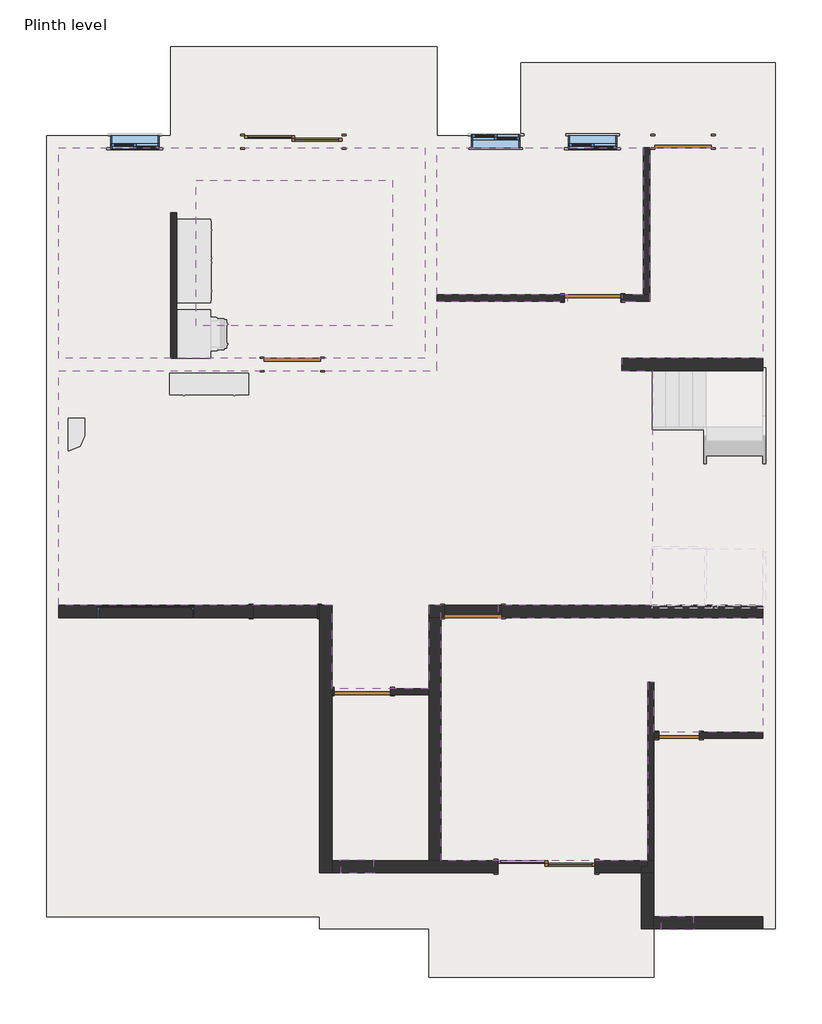
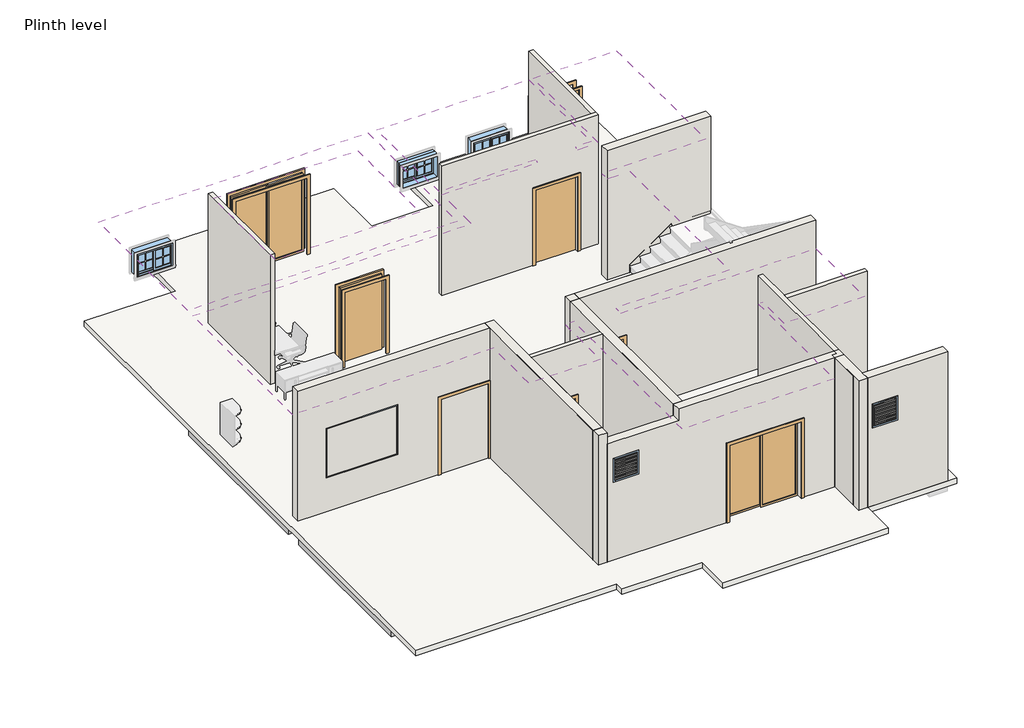
# One storey, part 1 of 2: 22 walls, 10 beams, 10 doors, 9 windows, 3 coverings, 1 slab.
"""IFC4 building model written with IfcOpenShell, lengths in millimetres."""

from ifc_helpers import new_model, si_unit, frame, origin, origin_with_axes, place, context, project, spatial, polyline, outline, extrude, faceted_brep, transform, mapped, element, save
from components import door_b7c0cbe2, door_d8f5dbb5, door_5f0ed9dd, door_edbf5142, door_f6232a3f, door_6982a541, window_dd9b4f56, window_f2d8fef0, window_5ed62b27

model = new_model("IFC4")

# Units and contexts
model_context = context("Model", 3, world=origin())
ifc_project = project(units=[si_unit("LENGTHUNIT", "METRE", prefix="MILLI")], contexts=[model_context])

# Site, building, storey
site = spatial("IfcSite", under=ifc_project)
building = spatial("IfcBuilding", under=site)
storey = spatial("IfcBuildingStorey", under=building, Name="Plinth level", Elevation=0.0)

# Beams
placement = place(None, origin())
element("IfcBeam", 1, ObjectType="Concrete-Rectangular Beam : 18X12", at=placement, inside=storey, context=model_context, shape_type="SweptSolid", body=[
    extrude(outline(polyline([(16230.9916032, -2769.6758122), (18402.6916032, -2769.6758122), (18402.6916032, -3226.8758122), (16688.1916032, -3226.8758122), (16688.1916032, -2998.2758122), (16230.9916032, -2998.2758122), (16230.9916032, -2769.6758122)])), frame((0.0, 0.0, -457.2), z_axis=(0.0, 0.0, 1.0), x_axis=(1.0, 0.0, 0.0)), (0.0, 0.0, 1.0), 304.8),
])
element("IfcBeam", 2, ObjectType="Concrete-Rectangular Beam : 18X12", at=placement, inside=storey, context=model_context, shape_type="Brep", body=[
    faceted_brep([(16230.9916032, -3226.8758122, -152.4), (16230.9916032, -2998.2758122, -152.4), (16230.9916032, -2769.6758122, -152.4), (12687.6916032, -2769.6758122, -152.4), (12687.6916032, -3226.8758122, -152.4), (16230.9916032, -3226.8758122, -457.2), (12687.6916032, -3226.8758122, -457.2), (16230.9916032, -2769.6758122, -457.2), (16230.9916032, -2998.2758122, -457.2), (12687.6916032, -2769.6758122, -457.2)], [[[0, 1, 2, 3, 4]], [[5, 0, 4, 6]], [[7, 8, 5, 6, 9]], [[2, 7, 9, 3]], [[3, 9, 6, 4]], [[2, 1, 0, 5, 8, 7]]]),
])
element("IfcBeam", 3, ObjectType="Concrete-Rectangular Beam : 18X12", at=placement, inside=storey, context=model_context, shape_type="Brep", body=[
    faceted_brep([(12459.0916032, -3226.8758122, -152.4), (12459.0916032, -2769.6758122, -152.4), (10858.8916032, -2769.6758122, -152.4), (10630.2916032, -2769.6758122, -152.4), (10630.2916032, -3226.8758122, -152.4), (12459.0916032, -2769.6758122, -457.2), (10858.8916032, -2769.6758122, -457.2), (10630.2916032, -2769.6758122, -457.2), (12459.0916032, -3226.8758122, -457.2), (10630.2916032, -3226.8758122, -457.2)], [[[0, 1, 2, 3, 4]], [[1, 5, 6, 7, 3, 2]], [[5, 8, 9, 7, 6]], [[8, 0, 4, 9]], [[0, 8, 5, 1]], [[4, 3, 7, 9]]]),
])
element("IfcBeam", 4, ObjectType="Concrete-Rectangular Beam : 18X12", at=placement, inside=storey, context=model_context, shape_type="Brep", body=[
    faceted_brep([(10858.8916032, -2769.6758122, -152.4), (10858.8916032, 1345.1241878, -152.4), (10858.8916032, 1802.3241878, -152.4), (10630.2916032, 1802.3241878, -152.4), (10630.2916032, 1345.1241878, -152.4), (10401.6916032, 1345.1241878, -152.4), (10401.6916032, -2769.6758122, -152.4), (10630.2916032, -2769.6758122, -152.4), (10858.8916032, 1802.3241878, -457.2), (10858.8916032, -2769.6758122, -457.2), (10858.8916032, 1345.1241878, -457.2), (10630.2916032, -2769.6758122, -457.2), (10401.6916032, -2769.6758122, -457.2), (10401.6916032, 1345.1241878, -457.2), (10630.2916032, 1345.1241878, -457.2), (10630.2916032, 1802.3241878, -457.2)], [[[0, 1, 2, 3, 4, 5, 6, 7]], [[8, 2, 1, 0, 9, 10]], [[8, 10, 9, 11, 12, 13, 14, 15]], [[12, 6, 5, 13]], [[0, 7, 6, 12, 11, 9]], [[2, 8, 15, 3]], [[14, 4, 3, 15]], [[4, 14, 13, 5]]]),
])
element("IfcBeam", 5, ObjectType="Concrete-Rectangular Beam : 18X12", at=placement, inside=storey, context=model_context, shape_type="Brep", body=[
    faceted_brep([(12459.0916032, 1345.1241878, -152.4), (12459.0916032, 1802.3241878, -152.4), (12153.8099466, 1802.3241878, -152.4), (10858.8916032, 1802.3241878, -152.4), (10858.8916032, 1345.1241878, -152.4), (12459.0916032, 1345.1241878, -457.2), (10858.8916032, 1345.1241878, -457.2), (12459.0916032, 1802.3241878, -457.2), (10858.8916032, 1802.3241878, -457.2), (12153.8099466, 1802.3241878, -457.2)], [[[0, 1, 2, 3, 4]], [[5, 0, 4, 6]], [[7, 5, 6, 8, 9]], [[1, 7, 9, 8, 3, 2]], [[4, 3, 8, 6]], [[1, 0, 5, 7]]]),
])
element("IfcBeam", 6, ObjectType="Concrete-Rectangular Beam : 18X12", at=placement, inside=storey, context=model_context, shape_type="Brep", body=[
    faceted_brep([(18402.6916032, 1345.1241878, -152.4), (18402.6916032, 1573.7241878, -152.4), (18402.6916032, 1802.3241878, -152.4), (12687.6916032, 1802.3241878, -152.4), (12687.6916032, 1345.1241878, -152.4), (18402.6916032, 1345.1241878, -457.2), (12687.6916032, 1345.1241878, -457.2), (18402.6916032, 1802.3241878, -457.2), (18402.6916032, 1573.7241878, -457.2), (12687.6916032, 1802.3241878, -457.2)], [[[0, 1, 2, 3, 4]], [[5, 0, 4, 6]], [[7, 8, 5, 6, 9]], [[2, 7, 9, 3]], [[3, 9, 6, 4]], [[2, 1, 0, 5, 8, 7]]]),
])
element("IfcBeam", 7, ObjectType="Concrete-Rectangular Beam : 18X12", at=placement, inside=storey, context=model_context, shape_type="Brep", body=[
    faceted_brep([(5601.0916032, 1802.3241878, -152.4), (5601.0916032, 1345.1241878, -152.4), (5829.6916032, 1345.1241878, -152.4), (10401.6916032, 1345.1241878, -152.4), (10401.6916032, 1802.3241878, -152.4), (5829.6916032, 1802.3241878, -152.4), (5601.0916032, 1345.1241878, -457.2), (5829.6916032, 1345.1241878, -457.2), (10401.6916032, 1345.1241878, -457.2), (5601.0916032, 1802.3241878, -457.2), (5829.6916032, 1802.3241878, -457.2), (10401.6916032, 1802.3241878, -457.2)], [[[0, 1, 2, 3, 4, 5]], [[1, 6, 7, 8, 3, 2]], [[6, 9, 10, 11, 8, 7]], [[9, 0, 5, 4, 11, 10]], [[1, 0, 9, 6]], [[4, 3, 8, 11]]]),
])
element("IfcBeam", 8, ObjectType="Concrete-Rectangular Beam : 18X12", at=placement, inside=storey, context=model_context, shape_type="Brep", body=[
    faceted_brep([(5601.0916032, -2769.6758122, -152.4), (5601.0916032, -3226.8758122, -152.4), (10401.6916032, -3226.8758122, -152.4), (10401.6916032, -2769.6758122, -152.4), (5829.6916032, -2769.6758122, -152.4), (5601.0916032, -3226.8758122, -457.2), (10401.6916032, -3226.8758122, -457.2), (5601.0916032, -2769.6758122, -457.2), (5829.6916032, -2769.6758122, -457.2), (10401.6916032, -2769.6758122, -457.2)], [[[0, 1, 2, 3, 4]], [[1, 5, 6, 2]], [[5, 7, 8, 9, 6]], [[7, 0, 4, 3, 9, 8]], [[1, 0, 7, 5]], [[3, 2, 6, 9]]]),
])
element("IfcBeam", 9, ObjectType="Concrete-Rectangular Beam : 18X12", at=placement, inside=storey, context=model_context, shape_type="Brep", body=[
    faceted_brep([(5829.6916032, 1345.1241878, -152.4), (5601.0916032, 1345.1241878, -152.4), (5372.4916032, 1345.1241878, -152.4), (5372.4916032, -2769.6758122, -152.4), (5601.0916032, -2769.6758122, -152.4), (5829.6916032, -2769.6758122, -152.4), (5829.6916032, 1345.1241878, -457.2), (5829.6916032, -2769.6758122, -457.2), (5372.4916032, 1345.1241878, -457.2), (5601.0916032, 1345.1241878, -457.2), (5601.0916032, -2769.6758122, -457.2), (5372.4916032, -2769.6758122, -457.2)], [[[0, 1, 2, 3, 4, 5]], [[6, 0, 5, 7]], [[8, 9, 6, 7, 10, 11]], [[2, 8, 11, 3]], [[2, 1, 0, 6, 9, 8]], [[5, 4, 3, 11, 10, 7]]]),
])
element("IfcBeam", 10, ObjectType="Concrete-Rectangular Beam : 18X12", at=placement, inside=storey, context=model_context, shape_type="Brep", body=[
    faceted_brep([(5829.6916032, 1802.3241878, -152.4), (5829.6916032, 6221.9241878, -152.4), (5829.6916032, 6679.1241878, -152.4), (5601.0916032, 6679.1241878, -152.4), (5601.0916032, 6221.9241878, -152.4), (5372.4916032, 6221.9241878, -152.4), (5372.4916032, 1802.3241878, -152.4), (5601.0916032, 1802.3241878, -152.4), (5372.4916032, 1802.3241878, -457.2), (5372.4916032, 6221.9241878, -457.2), (5829.6916032, 6679.1241878, -457.2), (5829.6916032, 6221.9241878, -457.2), (5829.6916032, 1802.3241878, -457.2), (5601.0916032, 1802.3241878, -457.2), (5601.0916032, 6221.9241878, -457.2), (5601.0916032, 6679.1241878, -457.2)], [[[0, 1, 2, 3, 4, 5, 6, 7]], [[8, 6, 5, 9]], [[10, 11, 12, 13, 8, 9, 14, 15]], [[10, 2, 1, 0, 12, 11]], [[0, 7, 6, 8, 13, 12]], [[2, 10, 15, 3]], [[14, 4, 3, 15]], [[4, 14, 9, 5]]]),
])

# Coverings
element("IfcCovering", 11, ObjectType="GWB on Mtl Stud", at=placement, inside=storey, context=model_context, shape_type="SweptSolid", body=[
    extrude(outline(polyline([(5486.7916032, 10412.9241878), (12382.4099466, 10412.9241878), (12382.4099466, 6450.5241878), (5486.7916032, 6450.5241878), (5486.7916032, 10412.9241878)]), holes=[polyline([(11772.8099466, 9803.3241878), (8077.5916032, 9803.3241878), (8077.5916032, 7060.1241878), (11772.8099466, 7060.1241878), (11772.8099466, 9803.3241878)])]), frame((0.0, 0.0, 2743.2), z_axis=(0.0, 0.0, 1.0), x_axis=(1.0, 0.0, 0.0)), (0.0, 0.0, 1.0), 107.95),
    extrude(outline(polyline([(11468.0099466, 9498.5241878), (11468.0099466, 7364.9241878), (8382.3916032, 7364.9241878), (8382.3916032, 9498.5241878), (11468.0099466, 9498.5241878)]), holes=[polyline([(11163.2099466, 9193.7241878), (8687.1916032, 9193.7241878), (8687.1916032, 8584.1241878), (11163.2099466, 8584.1241878), (11163.2099466, 9193.7241878)]), polyline([(8687.1916032, 8279.3241878), (8687.1916032, 7669.7241878), (11163.2099466, 7669.7241878), (11163.2099466, 8279.3241878), (8687.1916032, 8279.3241878)])]), frame((0.0, 0.0, 2743.2), z_axis=(0.0, 0.0, 1.0), x_axis=(1.0, 0.0, 0.0)), (0.0, 0.0, 1.0), 107.95),
])
element("IfcCovering", 12, ObjectType="GWB on Mtl Stud", at=placement, inside=storey, context=model_context, shape_type="SweptSolid", body=[
    extrude(outline(polyline([(11772.8099466, 9803.3241878), (11772.8099466, 7060.1241878), (8077.5916032, 7060.1241878), (8077.5916032, 9803.3241878), (11772.8099466, 9803.3241878)])), frame((0.0, 0.0, 2844.8), z_axis=(0.0, 0.0, 1.0), x_axis=(1.0, 0.0, 0.0)), (0.0, 0.0, 1.0), 107.95),
])
element("IfcCovering", 13, ObjectType="GWB on Mtl Stud", at=placement, inside=storey, context=model_context, shape_type="SweptSolid", body=[
    extrude(outline(polyline([(16497.2099466, 10412.9241878), (16497.2099466, 7644.3241878), (16086.4502792, 7644.3241878), (16086.4502792, 7530.0241878), (16611.5099466, 7530.0241878), (16611.5099466, 10412.9241878), (18745.5916032, 10412.9241878), (18745.5916032, 7530.0241878), (18745.5916032, 6450.5241878), (16086.4502792, 6450.5241878), (16086.4502792, 6221.9241878), (16662.7916032, 6221.9241878), (16662.7916032, 5155.1241878), (16662.7916032, 2869.1241878), (16662.7916032, 1802.3241878), (13751.6300735, 1802.3241878), (13751.6300735, 1573.7241878), (18745.5916032, 1573.7241878), (18745.5916032, -585.2758122), (16688.1916032, -585.2758122), (16688.1916032, 354.5241878), (16573.8916032, 354.5241878), (16573.8916032, -2998.2758122), (12687.6916032, -2998.2758122), (12687.6916032, 1802.3241878), (12459.0916032, 1802.3241878), (12459.0916032, 240.2241878), (10629.8628274, 240.2241878), (10629.8628274, 1802.3241878), (5486.7916032, 1802.3241878), (5486.7916032, 6221.9241878), (12611.0099466, 6221.9241878), (12611.0099466, 7530.0241878), (15070.4502792, 7530.0241878), (15070.4502792, 7644.3241878), (12611.0099466, 7644.3241878), (12611.0099466, 10412.9241878), (16497.2099466, 10412.9241878)])), frame((0.0, 0.0, 2743.2), z_axis=(0.0, 0.0, 1.0), x_axis=(1.0, 0.0, 0.0)), (0.0, 0.0, 1.0), 107.95),
])

# Doors
door_shape = door_b7c0cbe2(model_context)
element("IfcDoor", 14, ObjectType="Door-Double-Sliding : 72\" x 82\"", at=placement, inside=storey, context=model_context, shape_type="MappedRepresentation", body=[
    mapped(door_shape, transform((14668.8916032, -3239.5758122, 0.0), x_axis=(1.0, 0.0, 0.0), y_axis=(0.0, 1.0, 0.0), z_axis=(0.0, 0.0, 1.0))),
])
element("IfcDoor", 15, ObjectType="Door-Double-Sliding : 72\" x 82\"", at=placement, inside=storey, context=model_context, shape_type="MappedRepresentation", body=[
    mapped(door_shape, transform((9905.9099466, 10400.2241878, 0.0), x_axis=(1.0, 0.0, 0.0), y_axis=(0.0, 1.0, 0.0), z_axis=(0.0, 0.0, 1.0))),
])
element("IfcDoor", 16, ObjectType="Door-Double-Sliding : 72\" x 82\"", at=placement, inside=storey, context=model_context, shape_type="MappedRepresentation", body=[
    mapped(door_shape, transform((14668.8916032, -3239.5758122, 0.0), x_axis=(1.0, 0.0, 0.0), y_axis=(0.0, 1.0, 0.0), z_axis=(0.0, 0.0, 1.0))),
])
door_2_shape = door_d8f5dbb5(model_context)
element("IfcDoor", 17, ObjectType="Single-Flush : 30\" x 80\"", at=placement, inside=storey, context=model_context, shape_type="MappedRepresentation", body=[
    mapped(door_2_shape, transform((17164.4416032, -642.4258122, 0.0), x_axis=(-1.0, 0.0, 0.0), y_axis=(0.0, -1.0, 0.0), z_axis=(0.0, 0.0, 1.0))),
])
door_3_shape = door_5f0ed9dd(model_context)
element("IfcDoor", 18, ObjectType="Single-Flush : 42\" x 80\"", at=placement, inside=storey, context=model_context, shape_type="MappedRepresentation", body=[
    mapped(door_3_shape, transform((11201.7916032, 183.0741878, 0.0), x_axis=(-1.0, 0.0, 0.0), y_axis=(0.0, -1.0, 0.0), z_axis=(0.0, 0.0, 1.0))),
])
element("IfcDoor", 19, ObjectType="Single-Flush : 42\" x 80\"", at=placement, inside=storey, context=model_context, shape_type="MappedRepresentation", body=[
    mapped(door_3_shape, transform((15538.3599466, 7587.1741878, 0.0), x_axis=(1.0, 0.0, 0.0), y_axis=(0.0, 1.0, 0.0), z_axis=(0.0, 0.0, 1.0))),
])
door_4_shape = door_edbf5142(model_context)
element("IfcDoor", 20, ObjectType="Single-Flush : 42\" x 80\"", at=placement, inside=storey, context=model_context, shape_type="MappedRepresentation", body=[
    mapped(door_4_shape, transform((13284.5916032, 1688.0241878, 0.0), x_axis=(-1.0, 0.0, 0.0), y_axis=(0.0, -1.0, 0.0), z_axis=(0.0, 0.0, 1.0))),
])
element("IfcDoor", 21, ObjectType="Single-Flush : 42\" x 80\"", at=placement, inside=storey, context=model_context, shape_type="MappedRepresentation", body=[
    mapped(door_4_shape, transform((17240.1599466, 10527.2241878, 0.0), x_axis=(-1.0, 0.0, 0.0), y_axis=(0.0, -1.0, 0.0), z_axis=(0.0, 0.0, 1.0))),
])
door_5_shape = door_f6232a3f(model_context)
element("IfcDoor", 22, ObjectType="Single-Flush : 42\" x 80\"", at=placement, inside=storey, context=model_context, shape_type="MappedRepresentation", body=[
    mapped(door_5_shape, transform((9886.8599466, 6336.2241878, 0.0), x_axis=(-1.0, 0.0, 0.0), y_axis=(0.0, -1.0, 0.0), z_axis=(0.0, 0.0, 1.0))),
])
door_6_shape = door_6982a541(model_context)
element("IfcDoor", 23, ObjectType="Single-Flush : 48\" x 80\" 2", at=placement, inside=storey, context=model_context, shape_type="MappedRepresentation", body=[
    mapped(door_6_shape, transform((9753.9916032, 1688.0241878, 0.0), x_axis=(-1.0, 0.0, 0.0), y_axis=(0.0, -1.0, 0.0), z_axis=(0.0, 0.0, 1.0))),
])

# Slab
element("IfcSlab", 24, ObjectType="Concrete Slab - 6\"", at=placement, inside=storey, context=model_context, shape_type="SweptSolid", body=[
    extrude(outline(polyline([(5258.1916032, 10641.5241878), (7594.5099466, 10641.5241878), (7594.5099466, 12317.9241878), (12611.0099466, 12317.9241878), (12611.0099466, 10641.5241878), (14192.2689416, 10641.5241878), (14192.2689416, 12013.1241878), (18974.1916032, 12013.1241878), (18974.1916032, 10641.5241878), (18974.1916032, -4280.9758122), (16688.1916032, -4280.9758122), (16688.1916032, -5195.3758122), (12459.0916032, -5195.3758122), (12459.0916032, -4280.9758122), (10401.6916032, -4280.9758122), (10401.6916032, -4052.3758122), (5258.1916032, -4052.3758122), (5258.1916032, 10641.5241878)])), frame((0.0, 0.0, -152.4), z_axis=(0.0, 0.0, 1.0), x_axis=(1.0, 0.0, 0.0)), (0.0, 0.0, 1.0), 152.4),
])

# Walls
element("IfcWall", 25, ObjectType="4.5\"", at=placement, inside=storey, context=model_context, shape_type="Brep", body=[
    faceted_brep([(16688.1916032, -2998.2758122, 0.0), (16688.1916032, -699.5758122, 0.0), (16688.1916032, -585.2758122, 0.0), (16688.1916032, 354.5241878, 0.0), (16688.1916032, 354.5241878, 3505.2), (16688.1916032, -585.2758122, 3505.2), (16688.1916032, -699.5758122, 3505.2), (16688.1916032, -2998.2758122, 3505.2), (16573.8916032, -2998.2758122, 0.0), (16573.8916032, -2998.2758122, 3505.2), (16573.8916032, 354.5241878, 3505.2), (16573.8916032, 354.5241878, 0.0)], [[[0, 1, 2, 3, 4, 5, 6, 7]], [[8, 9, 10, 11]], [[3, 2, 1, 0, 8, 11]], [[4, 3, 11, 10]], [[7, 6, 5, 4, 10, 9]], [[0, 7, 9, 8]]]),
])
element("IfcWall", 26, ObjectType="4.5\"", at=placement, inside=storey, context=model_context, shape_type="SweptSolid", body=[
    extrude(outline(polyline([(0.0, 10630.2916032), (0.0, 10668.3916032), (2032.0, 10668.3916032), (2032.0, 11735.1916032), (0.0, 11735.1916032), (0.0, 12459.0916032), (3505.2, 12459.0916032), (3505.2, 10630.2916032), (0.0, 10630.2916032)])), frame((0.0, 125.9241878, 0.0), z_axis=(0.0, 1.0, 0.0), x_axis=(0.0, 0.0, 1.0)), (0.0, 0.0, 1.0), 114.3),
])
element("IfcWall", 27, ObjectType="4.5\"", at=placement, inside=storey, context=model_context, shape_type="SweptSolid", body=[
    extrude(outline(polyline([(7708.8099466, 9193.7241878), (7708.8099466, 6450.5241878), (7594.5099466, 6450.5241878), (7594.5099466, 9193.7241878), (7708.8099466, 9193.7241878)])), origin_with_axes(), (0.0, 0.0, 1.0), 3505.2),
])
element("IfcWall", 28, ObjectType="4.5\"", at=placement, inside=storey, context=model_context, shape_type="Brep", body=[
    faceted_brep([(16071.7599466, 7530.0241878, 2032.0), (16071.7599466, 7530.0241878, 0.0), (16611.5099466, 7530.0241878, 0.0), (16611.5099466, 7530.0241878, 3505.2), (12611.0099466, 7530.0241878, 3505.2), (12611.0099466, 7530.0241878, 0.0), (15004.9599466, 7530.0241878, 0.0), (15004.9599466, 7530.0241878, 2032.0), (16611.5099466, 7644.3241878, 0.0), (16497.2099466, 7644.3241878, 0.0), (16071.7599466, 7644.3241878, 0.0), (16071.7599466, 7644.3241878, 2032.0), (15004.9599466, 7644.3241878, 2032.0), (15004.9599466, 7644.3241878, 0.0), (12611.0099466, 7644.3241878, 0.0), (12611.0099466, 7644.3241878, 3505.2), (16497.2099466, 7644.3241878, 3505.2), (16611.5099466, 7644.3241878, 3505.2)], [[[0, 1, 2, 3, 4, 5, 6, 7]], [[8, 9, 10, 11, 12, 13, 14, 15, 16, 17]], [[6, 5, 14, 13]], [[2, 1, 10, 9, 8]], [[4, 3, 17, 16, 15]], [[5, 4, 15, 14]], [[3, 2, 8, 17]], [[11, 10, 1, 0]], [[12, 11, 0, 7]], [[13, 12, 7, 6]]]),
])
element("IfcWall", 29, ObjectType="4.5\"", at=placement, inside=storey, context=model_context, shape_type="SweptSolid", body=[
    extrude(outline(polyline([(16611.5099466, 10412.9241878), (16611.5099466, 7644.3241878), (16497.2099466, 7644.3241878), (16497.2099466, 10412.9241878), (16611.5099466, 10412.9241878)])), origin_with_axes(), (0.0, 0.0, 1.0), 3505.2),
])
element("IfcWall", 30, ObjectType="4.5\"", at=placement, inside=storey, context=model_context, shape_type="SweptSolid", body=[
    extrude(outline(polyline([(0.0, 16688.1916032), (0.0, 16783.4416032), (2032.0, 16783.4416032), (2032.0, 17545.4416032), (0.0, 17545.4416032), (0.0, 18745.5916032), (3505.2, 18745.5916032), (3505.2, 16688.1916032), (0.0, 16688.1916032)])), frame((0.0, -699.5758122, 0.0), z_axis=(0.0, 1.0, 0.0), x_axis=(0.0, 0.0, 1.0)), (0.0, 0.0, 1.0), 114.3),
])
element("IfcWall", 31, ObjectType="9\" wall", at=placement, inside=storey, context=model_context, shape_type="SweptSolid", body=[
    extrude(outline(polyline([(18745.5916032, 6221.9241878), (16086.4502792, 6221.9241878), (16086.4502792, 6450.5241878), (18745.5916032, 6450.5241878), (18745.5916032, 6221.9241878)])), origin_with_axes(), (0.0, 0.0, 1.0), 3505.2),
])
element("IfcWall", 32, ObjectType="9\" wall", at=placement, inside=storey, context=model_context, shape_type="Brep", body=[
    faceted_brep([(12751.1916032, 1802.3241878, 2032.0), (12751.1916032, 1802.3241878, 0.0), (12459.0916032, 1802.3241878, 0.0), (12459.0916032, 1802.3241878, 3505.2), (18745.5916032, 1802.3241878, 3505.2), (18745.5916032, 1802.3241878, 0.0), (13817.9916032, 1802.3241878, 0.0), (13817.9916032, 1802.3241878, 2032.0), (12459.0916032, 1573.7241878, 0.0), (12687.6916032, 1573.7241878, 0.0), (12751.1916032, 1573.7241878, 0.0), (12751.1916032, 1573.7241878, 2032.0), (13817.9916032, 1573.7241878, 2032.0), (13817.9916032, 1573.7241878, 0.0), (18745.5916032, 1573.7241878, 0.0), (18745.5916032, 1573.7241878, 3505.2), (12687.6916032, 1573.7241878, 3505.2), (12459.0916032, 1573.7241878, 3505.2)], [[[0, 1, 2, 3, 4, 5, 6, 7]], [[8, 9, 10, 11, 12, 13, 14, 15, 16, 17]], [[6, 5, 14, 13]], [[2, 1, 10, 9, 8]], [[4, 3, 17, 16, 15]], [[5, 4, 15, 14]], [[3, 2, 8, 17]], [[11, 10, 1, 0]], [[12, 11, 0, 7]], [[13, 12, 7, 6]]]),
])
element("IfcWall", 33, ObjectType="9\" wall", at=placement, inside=storey, context=model_context, shape_type="Brep", body=[
    faceted_brep([(12459.0916032, 1573.7241878, 0.0), (12459.0916032, 240.2241878, 0.0), (12459.0916032, 125.9241878, 0.0), (12459.0916032, -2998.2758122, 0.0), (12459.0916032, -2998.2758122, 3505.2), (12459.0916032, 125.9241878, 3505.2), (12459.0916032, 240.2241878, 3505.2), (12459.0916032, 1573.7241878, 3505.2), (12687.6916032, 1573.7241878, 0.0), (12687.6916032, 1573.7241878, 3505.2), (12687.6916032, -2998.2758122, 3505.2), (12687.6916032, -2998.2758122, 0.0)], [[[0, 1, 2, 3, 4, 5, 6, 7]], [[8, 9, 10, 11]], [[3, 2, 1, 0, 8, 11]], [[7, 6, 5, 4, 10, 9]], [[0, 7, 9, 8]], [[4, 3, 11, 10]]]),
])
element("IfcWall", 34, ObjectType="9\" wall", at=placement, inside=storey, context=model_context, shape_type="Brep", body=[
    faceted_brep([(10630.2916032, -3226.8758122, 0.0), (10630.2916032, -2998.2758122, 0.0), (10630.2916032, 125.9241878, 0.0), (10630.2916032, 240.2241878, 0.0), (10630.2916032, 1802.3241878, 0.0), (10630.2916032, 1802.3241878, 3505.2), (10630.2916032, 240.2241878, 3505.2), (10630.2916032, 125.9241878, 3505.2), (10630.2916032, -2998.2758122, 3505.2), (10630.2916032, -3226.8758122, 3505.2), (10401.6916032, -3226.8758122, 0.0), (10401.6916032, -3226.8758122, 3505.2), (10401.6916032, 1573.7241878, 3505.2), (10401.6916032, 1802.3241878, 3505.2), (10401.6916032, 1802.3241878, 0.0), (10401.6916032, 1573.7241878, 0.0)], [[[0, 1, 2, 3, 4, 5, 6, 7, 8, 9]], [[10, 11, 12, 13, 14, 15]], [[4, 3, 2, 1, 0, 10, 15, 14]], [[9, 8, 7, 6, 5, 13, 12, 11]], [[0, 9, 11, 10]], [[5, 4, 14, 13]]]),
])
element("IfcWall", 35, ObjectType="9\" wall", at=placement, inside=storey, context=model_context, shape_type="SweptSolid", body=[
    extrude(outline(polyline([(16688.1916032, -2998.2758122), (16688.1916032, -3226.8758122), (16459.5916032, -3226.8758122), (16459.5916032, -3112.5758122), (16573.8916032, -3112.5758122), (16573.8916032, -2998.2758122), (16688.1916032, -2998.2758122)])), origin_with_axes(), (0.0, 0.0, 1.0), 3505.2),
])
element("IfcWall", 36, ObjectType="9\" wall", at=placement, inside=storey, context=model_context, shape_type="Brep", body=[
    faceted_brep([(16459.5916032, -3226.8758122, 0.0), (16459.5916032, -4280.9758122, 0.0), (16459.5916032, -4280.9758122, 3505.2), (16459.5916032, -3226.8758122, 3505.2), (16688.1916032, -3226.8758122, 0.0), (16688.1916032, -3226.8758122, 3505.2), (16688.1916032, -4052.3758122, 3505.2), (16688.1916032, -4280.9758122, 3505.2), (16688.1916032, -4280.9758122, 0.0), (16688.1916032, -4052.3758122, 0.0)], [[[0, 1, 2, 3]], [[4, 5, 6, 7, 8, 9]], [[1, 0, 4, 9, 8]], [[3, 2, 7, 6, 5]], [[0, 3, 5, 4]], [[2, 1, 8, 7]]]),
])
element("IfcWall", 37, ObjectType="9\" wall", at=placement, inside=storey, context=model_context, shape_type="SweptSolid", body=[
    extrude(outline(polyline([(0.0, 16688.1916032), (0.0, 18745.5916032), (3505.2, 18745.5916032), (3505.2, 16688.1916032), (0.0, 16688.1916032)]), holes=[polyline([(2743.2, 17437.4916032), (2133.6, 17437.4916032), (2133.6, 16827.8916032), (2743.2, 16827.8916032), (2743.2, 17437.4916032)])]), frame((0.0, -4280.9758122, 0.0), z_axis=(0.0, 1.0, 0.0), x_axis=(0.0, 0.0, 1.0)), (0.0, 0.0, 1.0), 228.6),
])
element("IfcWall", 38, ObjectType="9\" wall", at=placement, inside=storey, context=model_context, shape_type="SweptSolid", body=[
    extrude(outline(polyline([(0.0, 5486.7916032), (0.0, 9144.3916032), (2032.0, 9144.3916032), (2032.0, 10363.5916032), (0.0, 10363.5916032), (0.0, 10401.6916032), (3505.2, 10401.6916032), (3505.2, 5486.7916032), (0.0, 5486.7916032)]), holes=[polyline([(2260.6, 8039.4916032), (914.4, 8039.4916032), (914.4, 6210.6916032), (2260.6, 6210.6916032), (2260.6, 8039.4916032)])]), frame((0.0, 1573.7241878, 0.0), z_axis=(0.0, 1.0, 0.0), x_axis=(0.0, 0.0, 1.0)), (0.0, 0.0, 1.0), 228.6),
])
element("IfcWall", 39, ObjectType="9\" wall", at=placement, inside=storey, context=model_context, shape_type="SweptSolid", body=[
    extrude(outline(polyline([(18745.5916032, 6221.9241878), (16086.4502792, 6221.9241878), (16086.4502792, 6450.5241878), (18745.5916032, 6450.5241878), (18745.5916032, 6221.9241878)])), origin_with_axes(), (0.0, 0.0, 1.0), 3505.2),
])
element("IfcWall", 40, ObjectType="9\" wall", at=placement, inside=storey, context=model_context, shape_type="SweptSolid", body=[
    extrude(outline(polyline([(12687.6916032, 1802.3241878), (18745.5916032, 1802.3241878), (18745.5916032, 1573.7241878), (12687.6916032, 1573.7241878), (12687.6916032, 1802.3241878)])), origin_with_axes(), (0.0, 0.0, 1.0), 3505.2),
])
element("IfcWall", 41, ObjectType="9\" wall", at=placement, inside=storey, context=model_context, shape_type="SweptSolid", body=[
    extrude(outline(polyline([(12459.0916032, -2998.2758122), (12459.0916032, 1573.7241878), (12687.6916032, 1573.7241878), (12687.6916032, -2998.2758122), (12459.0916032, -2998.2758122)])), origin_with_axes(), (0.0, 0.0, 1.0), 3505.2),
])
element("IfcWall", 42, ObjectType="9\" wall", at=placement, inside=storey, context=model_context, shape_type="SweptSolid", body=[
    extrude(outline(polyline([(10630.2916032, 1573.7241878), (10630.2916032, -2998.2758122), (10401.6916032, -2998.2758122), (10401.6916032, 1573.7241878), (10630.2916032, 1573.7241878)])), origin_with_axes(), (0.0, 0.0, 1.0), 3505.2),
])
element("IfcWall", 43, ObjectType="9\" wall", at=placement, inside=storey, context=model_context, shape_type="Brep", body=[
    faceted_brep([(13754.4916032, -3226.8758122, 0.0), (13754.4916032, -3226.8758122, 2082.8), (15583.2916032, -3226.8758122, 2082.8), (15583.2916032, -3226.8758122, 0.0), (16459.5916032, -3226.8758122, 0.0), (16459.5916032, -3226.8758122, 3505.2), (12459.0916032, -3226.8758122, 3505.2), (12459.0916032, -3226.8758122, 3200.4), (10630.2916032, -3226.8758122, 3200.4), (10630.2916032, -3226.8758122, 0.0), (16573.8916032, -2998.2758122, 3505.2), (16573.8916032, -2998.2758122, 0.0), (15583.2916032, -2998.2758122, 0.0), (15583.2916032, -2998.2758122, 2082.8), (13754.4916032, -2998.2758122, 2082.8), (13754.4916032, -2998.2758122, 0.0), (12687.6916032, -2998.2758122, 0.0), (12459.0916032, -2998.2758122, 0.0), (10630.2916032, -2998.2758122, 0.0), (10630.2916032, -2998.2758122, 3200.4), (12459.0916032, -2998.2758122, 3200.4), (12459.0916032, -2998.2758122, 3505.2), (12687.6916032, -2998.2758122, 3505.2), (16573.8916032, -3112.5758122, 0.0), (16459.5916032, -3112.5758122, 0.0), (16573.8916032, -3112.5758122, 3505.2), (16459.5916032, -3112.5758122, 3505.2)], [[[0, 1, 2, 3, 4, 5, 6, 7, 8, 9]], [[10, 11, 12, 13, 14, 15, 16, 17, 18, 19, 20, 21, 22]], [[15, 0, 9, 18, 17, 16]], [[3, 12, 11, 23, 24, 4]], [[25, 10, 22, 21, 6, 5, 26]], [[15, 14, 1, 0]], [[13, 12, 3, 2]], [[14, 13, 2, 1]], [[18, 9, 8, 19]], [[5, 4, 24, 26]], [[24, 23, 25, 26]], [[11, 10, 25, 23]], [[7, 20, 19, 8]], [[20, 7, 6, 21]]]),
])
element("IfcWall", 44, ObjectType="9\" wall", at=placement, inside=storey, context=model_context, shape_type="SweptSolid", body=[
    extrude(outline(polyline([(16459.5916032, -4052.3758122), (16459.5916032, -3226.8758122), (16688.1916032, -3226.8758122), (16688.1916032, -4052.3758122), (16459.5916032, -4052.3758122)])), origin_with_axes(), (0.0, 0.0, 1.0), 3505.2),
])
element("IfcWall", 45, ObjectType="9\" wall", at=placement, inside=storey, context=model_context, shape_type="SweptSolid", body=[
    extrude(outline(polyline([(18745.5916032, -4280.9758122), (16688.1916032, -4280.9758122), (16688.1916032, -4052.3758122), (18745.5916032, -4052.3758122), (18745.5916032, -4280.9758122)])), origin_with_axes(), (0.0, 0.0, 1.0), 3505.2),
])
element("IfcWall", 46, ObjectType="9\" wall", at=placement, inside=storey, context=model_context, shape_type="SweptSolid", body=[
    extrude(outline(polyline([(5486.7916032, 1802.3241878), (10401.6916032, 1802.3241878), (10401.6916032, 1573.7241878), (5486.7916032, 1573.7241878), (5486.7916032, 1802.3241878)])), origin_with_axes(), (0.0, 0.0, 1.0), 3505.2),
])

# Windows
window_shape = window_dd9b4f56(model_context)
element("IfcWindow", 47, ObjectType="Window-Awning-Variable : 72\" x 53\"", at=placement, inside=storey, context=model_context, shape_type="MappedRepresentation", body=[
    mapped(window_shape, transform((7125.0916032, 1688.0241878, 0.0), x_axis=(1.0, 0.0, 0.0), y_axis=(0.0, 1.0, 0.0), z_axis=(0.0, 0.0, 1.0))),
])
window_2_shape = window_f2d8fef0(model_context)
element("IfcWindow", 48, ObjectType="Window-Louvers : 24\" x 24\"", at=placement, inside=storey, context=model_context, shape_type="MappedRepresentation", body=[
    mapped(window_2_shape, transform((11106.5416032, -3118.9258122, 1219.2), x_axis=(-1.0, 0.0, 0.0), y_axis=(0.0, -1.0, 0.0), z_axis=(0.0, 0.0, 1.0))),
])
element("IfcWindow", 49, ObjectType="Window-Louvers : 24\" x 24\"", at=placement, inside=storey, context=model_context, shape_type="MappedRepresentation", body=[
    mapped(window_2_shape, transform((17132.6916032, -4173.0258122, 1219.2), x_axis=(-1.0, 0.0, 0.0), y_axis=(0.0, -1.0, 0.0), z_axis=(0.0, 0.0, 1.0))),
])
window_3_shape = window_5ed62b27(model_context)
element("IfcWindow", 50, ObjectType="Window-Sliding-Double : 36\" x 24\"", at=placement, inside=storey, context=model_context, shape_type="MappedRepresentation", body=[
    mapped(window_3_shape, transform((6921.8916032, 10523.4141878, 0.0), x_axis=(-1.0, 0.0, 0.0), y_axis=(0.0, -1.0, 0.0), z_axis=(0.0, 0.0, 1.0))),
])
element("IfcWindow", 51, ObjectType="Window-Sliding-Double : 36\" x 24\"", at=placement, inside=storey, context=model_context, shape_type="MappedRepresentation", body=[
    mapped(window_3_shape, transform((13715.9099466, 10531.0341878, 0.0), x_axis=(1.0, 0.0, 0.0), y_axis=(0.0, 1.0, 0.0), z_axis=(0.0, 0.0, 1.0))),
])
element("IfcWindow", 52, ObjectType="Window-Sliding-Double : 36\" x 24\"", at=placement, inside=storey, context=model_context, shape_type="MappedRepresentation", body=[
    mapped(window_3_shape, transform((15538.3599466, 10523.4141878, 0.0), x_axis=(-1.0, 0.0, 0.0), y_axis=(0.0, -1.0, 0.0), z_axis=(0.0, 0.0, 1.0))),
])
element("IfcWindow", 53, ObjectType="Window-Sliding-Double : 36\" x 24\"", at=placement, inside=storey, context=model_context, shape_type="MappedRepresentation", body=[
    mapped(window_3_shape, transform((6921.8916032, 10523.4141878, 0.0), x_axis=(-1.0, 0.0, 0.0), y_axis=(0.0, -1.0, 0.0), z_axis=(0.0, 0.0, 1.0))),
])
element("IfcWindow", 54, ObjectType="Window-Sliding-Double : 36\" x 24\"", at=placement, inside=storey, context=model_context, shape_type="MappedRepresentation", body=[
    mapped(window_3_shape, transform((13715.9099466, 10531.0341878, 0.0), x_axis=(1.0, 0.0, 0.0), y_axis=(0.0, 1.0, 0.0), z_axis=(0.0, 0.0, 1.0))),
])
element("IfcWindow", 55, ObjectType="Window-Sliding-Double : 36\" x 24\"", at=placement, inside=storey, context=model_context, shape_type="MappedRepresentation", body=[
    mapped(window_3_shape, transform((15538.3599466, 10523.4141878, 0.0), x_axis=(-1.0, 0.0, 0.0), y_axis=(0.0, -1.0, 0.0), z_axis=(0.0, 0.0, 1.0))),
])

save(model, "model.ifc")

# Revit data of these elements
# Type "Concrete-Rectangular Beam : 18X12"
#   Assembly Code = "B10"
#   Length [instance default] = 5' - 0"
#   b = 1' - 6"
#   h = 1' - 0"
#   Structural Material [instance default] = Concrete, Cast-in-Place gray
# Type "GWB on Mtl Stud"
#   Assembly Code = "C3030220"
#   built-in parameter 1002203 = 1 (stored number, unit not read)
#   built-in parameter 1002202 = 1 (stored number, unit not read)
#   Layers, outside or top first: 0' - 3 5/8" "Metal Stud Layer" (function 1); 0' - 0 5/8" "Gypsum Wall Board" (function 5)
# Type "Door-Double-Sliding : 72\" x 82\""
#   Type Mark = "17"
#   Construction Type Id = "opn-d45"
#   Assembly Code = "C1020"
#   Analytic Construction = "Wood frame, double glass door "
#   Thickness = 0' - 2"
#   Thermal Resistance (R) = 1.8150 (h·ft²·°F)/BTU
#   Heat Transfer Coefficient (U) = 0.5510 BTU/(h·ft²·°F)
#   Height = 6' - 10"
#   Rail Width = 0' - 2"
#   Stiles = 0' - 2"
#   Trim Projection Ext = 0' - 1"
#   Trim Projection Int = 0' - 1"
#   Trim Width = 0' - 3"
#   Width = 6' - 0"
#   Define Thermal Properties by = 1
#   Glazing = Glass
#   Panel Material = Wood - Birch - Solid Stained Light Low Gloss
#   Trim Material = Paint - Sienna
#   Visual Light Transmittance = 0
#   Solar Heat Gain Coefficient = 0
#   Function = (empty or 0)
#   Wall Closure = (empty or 0)
# Type "Single-Flush : 30\" x 80\""
#   Type Mark = "12"
#   Construction Type Id = "MDOOR"
#   Assembly Code = "C1020"
#   Analytic Construction = "Metal"
#   Thickness = 0' - 2"
#   Heat Transfer Coefficient (U) = 0.651978 BTU/(h·ft²·°F)
#   Height = 6' - 8"
#   Trim Projection Ext = 0' - 1"
#   Trim Projection Int = 0' - 1"
#   Trim Width = 0' - 3"
#   Width = 2' - 6"
#   Define Thermal Properties by = 1
#   Define Thermal Properties by = 1
#   Door Material = Door - Panel
#   Frame Material = Door - Frame
#   Visual Light Transmittance = 0
#   Solar Heat Gain Coefficient = 0
#   Function = (empty or 0)
#   Wall Closure = (empty or 0)
# Type "Single-Flush : 42\" x 80\""
#   Type Mark = "15"
#   Construction Type Id = "MDOOR"
#   Assembly Code = "C1020"
#   Analytic Construction = "Metal"
#   Thickness = 0' - 2"
#   Heat Transfer Coefficient (U) = 0.651978 BTU/(h·ft²·°F)
#   Height = 6' - 8"
#   Trim Projection Ext = 0' - 1"
#   Trim Projection Int = 0' - 1"
#   Trim Width = 0' - 3"
#   Width = 3' - 6"
#   Define Thermal Properties by = 1
#   Door Material = Door - Panel
#   Frame Material = Door - Frame
#   Visual Light Transmittance = 0
#   Solar Heat Gain Coefficient = 0
#   Function = (empty or 0)
#   Wall Closure = (empty or 0)
# Type "Single-Flush : 48\" x 80\" 2"
#   Type Mark = "16"
#   Construction Type Id = "MDOOR"
#   Assembly Code = "C1020"
#   Analytic Construction = "Metal"
#   Thickness = 0' - 2"
#   Heat Transfer Coefficient (U) = 0.651978 BTU/(h·ft²·°F)
#   Height = 6' - 8"
#   Trim Projection Ext = 0' - 1"
#   Trim Projection Int = 0' - 1"
#   Trim Width = 0' - 3"
#   Width = 4' - 0"
#   Define Thermal Properties by = 1
#   Door Material = Door - Panel
#   Frame Material = Door - Frame
#   Visual Light Transmittance = 0
#   Solar Heat Gain Coefficient = 0
#   Function = (empty or 0)
#   Wall Closure = (empty or 0)
# Type "Concrete Slab - 6\""
#   Assembly Code = "B1010"
#   Function = 0
#   Layers, outside or top first: 0' - 6" "Concrete, Cast-in-Place gray" (function 1)
# Type "4.5\""
#   Assembly Code = "B2010"
#   Layers, outside or top first: 0' - 4 1/2" no material (function 1)
# Type "9\" wall"
#   Assembly Code = "B2010"
#   Layers, outside or top first: 0' - 9" no material (function 1)
# Type "Window-Awning-Variable : 72\" x 53\""
#   Type Mark = "39"
#   Fire Rating = "0.5h"
#   Assembly Code = "B2020100"
#   Analytic Construction = "Double glazing - domestic"
#   Window Inset [instance default] = 0' - 0 5/8"
#   Wall Thickness [instance default] = 0' - 6"
#   Visual Light Transmittance = 0.81
#   Transom Height Ratio = 0.3
#   Transom Height = 1' - 3.9"
#   Thermal Resistance (R) = 1.8146 (h·ft²·°F)/BTU
#   Solar Heat Gain Coefficient = 0.76
#   Rough Width = 6' - 0 1/2"
#   Rough Height = 4' - 5 1/2"
#   Opening Window Width = 4' - 0"
#   Opening Window Height = 1' - 9.2"
#   Heat Transfer Coefficient (U) = 0.5511 BTU/(h·ft²·°F)
#   Height = 4' - 5"
#   Frame Gap 3 [instance default] = 0' - 1 83/128"
#   Frame Gap 2 [instance default] = 0' - 0 5/8"
#   Frame Gap 1 = 0' - 1 51/128"
#   Fixed Window Width = 2' - 0"
#   Default Sill Height = 3' - 0"
#   Width = 6' - 0"
#   Frame Material = Metal - Aluminum
#   Glass Panel Material = Glass
#   Wall Closure = (empty or 0)
# Type "Window-Louvers : 24\" x 24\""
#   Type Mark = "42"
#   Construction Type Id = "GSP4R"
#   Assembly Code = "B20"
#   Analytic Construction = "1/8 in Pilkington single glazing"
#   Visual Light Transmittance = 0.9
#   Thermal Resistance (R) = 1.53941 (h·ft²·°F)/BTU
#   Solar Heat Gain Coefficient = 0.78
#   Max Height = 1' - 11.74264"
#   Height = 2' - 0"
#   Heat Transfer Coefficient (U) = 0.6496 BTU/(h·ft²·°F)
#   Blade Width [instance default] = 1' - 10 1/2"
#   Blade Vertical Thickness = 0' - 0.35355"
#   Blade Thickness = 0' - 0 1/4"
#   Blade Spacing = 0' - 1 1/2"
#   Blade Height = 0' - 1.85355"
#   Blade Depth = 0' - 3"
#   Blade Angle = 45.00°
#   Default Sill Height = 3' - 0"
#   Trim Projection_Exterior = 0' - 0 1/2"
#   Trim Projection_Interior = 0' - 0 1/2"
#   Trim Width_Exterior = 0' - 1 1/2"
#   Trim Width_Interior = 0' - 1 1/2"
#   Width = 2' - 0"
#   Max Blade Count = 12
#   Define Thermal Properties by = 1
#   Blade Count = 12
#   Frame Material = Birch
#   Louver Material = Birch
#   Trim Exterior Material = Birch
#   Trim Interior Material = Birch
#   Wall Closure = (empty or 0)
# Type "Window-Sliding-Double : 36\" x 24\""
#   Type Mark = "27"
#   Fire Rating = "0.5h"
#   Assembly Code = "B2020100"
#   Analytic Construction = "Double glazing - domestic"
#   Window Inset [instance default] = 0' - 0"
#   Wall Thickness [instance default] = 0' - 6"
#   Visual Light Transmittance = 0.81
#   Thermal Resistance (R) = 1.8146 (h·ft²·°F)/BTU
#   Solar Heat Gain Coefficient = 0.76
#   Muntin Width = 1' - 2 5/8"
#   Muntin Height = 1' - 6 1/4"
#   Interior Wall Closure [instance default] = 0' - 2 3/4"
#   Heat Transfer Coefficient (U) = 0.5511 BTU/(h·ft²·°F)
#   Frame Extension [instance default] = 0' - 0 1/4"
#   Exterior Wall Closure [instance default] = 0' - 1 1/4"
#   Rough Width = 3' - 0 1/2"
#   Rough Height = 2' - 0 1/2"
#   Height = 2' - 0"
#   Extension Jamb [instance default] = 0' - 2 3/4"
#   Default Sill Height = 3' - 0"
#   Width = 3' - 0"
#   Interior Trim Visibility [instance default] = yes
#   Indicator Visibility [instance default] = yes
#   Exterior Trim Visibility [instance default] = yes
#   Muntin Visibility = yes
#   Extension Jamb Visibility [instance default] = yes
#   Muntin Pattern = Muntin Pattern_2x2 : Muntin Pattern_2x2
#   Interior Trim Material = Wood - Stained
#   Interior Trim = Trim-Window-Interior-Flat : Picture Frame
#   Interior Frame Material = Wood - Stained
#   Glass Panel Material = Glass
#   Exterior Trim Material = Clad - White
#   Exterior Trim = Trim-Window-Exterior-Flat : with Sill
#   Exterior Frame Material = Clad - White
#   Wall Closure = (empty or 0)
# Elements 1, 2, 3, 4, 5, 6, 7, 8, 9, 10 (IfcBeam, "Concrete-Rectangular Beam : 18X12")
#   Structural Material = Concrete, Cast-in-Place gray
#   Phase Created = Project Completion
#   Materials on its faces: "Concrete, Cast-in-Place gray"
# Elements 11, 13 (IfcCovering, "GWB on Mtl Stud")
#   Height Offset From Level = 9' - 0"
#   Phase Created = A10 - Substructure
#   Materials on its faces: "Gypsum Wall Board", "Metal Stud Layer"
# Element 12 (IfcCovering, "GWB on Mtl Stud")
#   Height Offset From Level = 9' - 4"
#   Phase Created = A10 - Substructure
#   Materials on its faces: "Gypsum Wall Board", "Metal Stud Layer"
# Elements 14, 15, 16 (IfcDoor, "Door-Double-Sliding : 72\" x 82\"")
#   Phase Created = Project Completion
#   Materials on its faces: "Paint - Sienna", "Wood - Birch - Solid Stained Light Low Gloss", "Glass"
# Element 17 (IfcDoor, "Single-Flush : 30\" x 80\"")
#   Phase Created = Project Completion
#   Materials on its faces: "Door - Frame", "Door - Panel"
# Elements 18, 19, 20, 21, 22 (IfcDoor, "Single-Flush : 42\" x 80\"")
#   Phase Created = Project Completion
#   Materials on its faces: "Door - Frame", "Door - Panel"
# Element 23 (IfcDoor, "Single-Flush : 48\" x 80\" 2")
#   Phase Created = Project Completion
#   Materials on its faces: "Door - Frame", "Door - Panel"
# Element 24 (IfcSlab, "Concrete Slab - 6\"")
#   Height Offset From Level = 0' - 0"
#   Phase Created = Project Completion
#   Materials on its faces: "Concrete, Cast-in-Place gray"
# Elements 25, 26, 27, 28, 29, 30 (IfcWall, "4.5\"")
#   Top Offset = 0' - 0"
#   Base Offset = 0' - 0"
#   wall height = 11' - 6"
#   Phase Created = Project Completion
#   Base Constraint = Plinth level
#   Top Constraint = FF
#   Materials on its faces: "Default Wall"
# Elements 31, 32, 33, 34, 35, 36, 37, 38, 39, 40, 41, 42, 43, 44, 45, 46 (IfcWall, "9\" wall")
#   Top Offset = 0' - 0"
#   Base Offset = 0' - 0"
#   wall height = 11' - 6"
#   Phase Created = Project Completion
#   Base Constraint = Plinth level
#   Top Constraint = FF
#   Materials on its faces: "Default Wall"
# Element 47 (IfcWindow, "Window-Awning-Variable : 72\" x 53\"")
#   Mark = "6"
#   Window Inset = 0' - 0 5/8"
#   Frame Gap 3 = 0' - 1 83/128"
#   Frame Gap 2 = 0' - 0 5/8"
#   Phase Created = Project Completion
#   Materials on its faces: "Glass", "Metal - Aluminum"
# Element 48 (IfcWindow, "Window-Louvers : 24\" x 24\"")
#   Mark = "7"
#   Blade Width = 1' - 10 1/2"
#   Phase Created = Project Completion
#   Materials on its faces: "Birch"
# Element 49 (IfcWindow, "Window-Louvers : 24\" x 24\"")
#   Mark = "8"
#   Blade Width = 1' - 10 1/2"
#   Phase Created = Project Completion
#   Materials on its faces: "Birch"
# Element 50 (IfcWindow, "Window-Sliding-Double : 36\" x 24\"")
#   Mark = "1"
#   Window Inset = 0' - 0"
#   Interior Wall Closure = 0' - 2 3/4"
#   Frame Extension = 0' - 0 1/4"
#   Exterior Wall Closure = 0' - 1 1/4"
#   Interior Trim Visibility = yes
#   Indicator Visibility = yes
#   Exterior Trim Visibility = yes
#   Phase Created = Project Completion
#   Materials on its faces: "Wood - Stained", "Glass", "Clad - White"
# Element 51 (IfcWindow, "Window-Sliding-Double : 36\" x 24\"")
#   Mark = "2"
#   Window Inset = 0' - 0"
#   Interior Wall Closure = 0' - 2 3/4"
#   Frame Extension = 0' - 0 1/4"
#   Exterior Wall Closure = 0' - 1 1/4"
#   Interior Trim Visibility = yes
#   Indicator Visibility = yes
#   Exterior Trim Visibility = yes
#   Phase Created = Project Completion
#   Materials on its faces: "Wood - Stained", "Glass", "Clad - White"
# Element 52 (IfcWindow, "Window-Sliding-Double : 36\" x 24\"")
#   Mark = "3"
#   Window Inset = 0' - 0"
#   Interior Wall Closure = 0' - 2 3/4"
#   Frame Extension = 0' - 0 1/4"
#   Exterior Wall Closure = 0' - 1 1/4"
#   Interior Trim Visibility = yes
#   Indicator Visibility = yes
#   Exterior Trim Visibility = yes
#   Phase Created = Project Completion
#   Materials on its faces: "Wood - Stained", "Glass", "Clad - White"
# Element 53 (IfcWindow, "Window-Sliding-Double : 36\" x 24\"")
#   Mark = "9"
#   Window Inset = 0' - 0"
#   Interior Wall Closure = 0' - 2 3/4"
#   Frame Extension = 0' - 0 1/4"
#   Exterior Wall Closure = 0' - 1 1/4"
#   Interior Trim Visibility = yes
#   Indicator Visibility = yes
#   Exterior Trim Visibility = yes
#   Phase Created = Project Completion
#   Materials on its faces: "Wood - Stained", "Glass", "Clad - White"
# Element 54 (IfcWindow, "Window-Sliding-Double : 36\" x 24\"")
#   Mark = "10"
#   Window Inset = 0' - 0"
#   Interior Wall Closure = 0' - 2 3/4"
#   Frame Extension = 0' - 0 1/4"
#   Exterior Wall Closure = 0' - 1 1/4"
#   Interior Trim Visibility = yes
#   Indicator Visibility = yes
#   Exterior Trim Visibility = yes
#   Phase Created = Project Completion
#   Materials on its faces: "Wood - Stained", "Glass", "Clad - White"
# Element 55 (IfcWindow, "Window-Sliding-Double : 36\" x 24\"")
#   Mark = "11"
#   Window Inset = 0' - 0"
#   Interior Wall Closure = 0' - 2 3/4"
#   Frame Extension = 0' - 0 1/4"
#   Exterior Wall Closure = 0' - 1 1/4"
#   Interior Trim Visibility = yes
#   Indicator Visibility = yes
#   Exterior Trim Visibility = yes
#   Phase Created = Project Completion
#   Materials on its faces: "Wood - Stained", "Glass", "Clad - White"
# Materials
#   "Concrete, Cast-in-Place gray": class "Concrete", colour RGB 192 192 192, transparency 0, Description = "Cast-in-place concrete", Cost = 0
#   "Metal Stud Layer": class "Metal", colour RGB 199 199 199, transparency 0, Description = "Light gauge steel framing, thermal air layer", Cost = 0
#   "Gypsum Wall Board": class "Generic", colour RGB 127 127 127, transparency 0, Description = "Gypsum Wall Board", Cost = 0
#   "Glass": class "Glass", colour RGB 0 128 192, transparency 0.75, Description = "Soda Lime Glass", Cost = 0
#   "Wood - Birch - Solid Stained Light Low Gloss": class "Wood", colour RGB 210 159 95, transparency 0, Cost = 0
#   "Paint - Sienna": colour RGB 118 70 51, transparency 0, Cost = 0
#   "Door - Panel": class "Wood", colour RGB 210 159 95, transparency 0, Cost = 0
#   "Door - Frame": colour RGB 118 70 51, transparency 0, Cost = 0
#   "Metal - Aluminum": class "Metal", colour RGB 247 247 247, transparency 0
#   "Birch": class "Wood", colour RGB 224 178 126, transparency 0, Description = "Betula Alleghaniensis", Cost = 0
#   "Wood - Stained": class "Wood", colour RGB 224 178 126, transparency 0, Cost = 0
#   "Clad - White": class "Wood", colour RGB 0 0 0, transparency 0, Cost = 0
#   "Default Wall": colour RGB 128 128 128, transparency 0, Cost = 0
